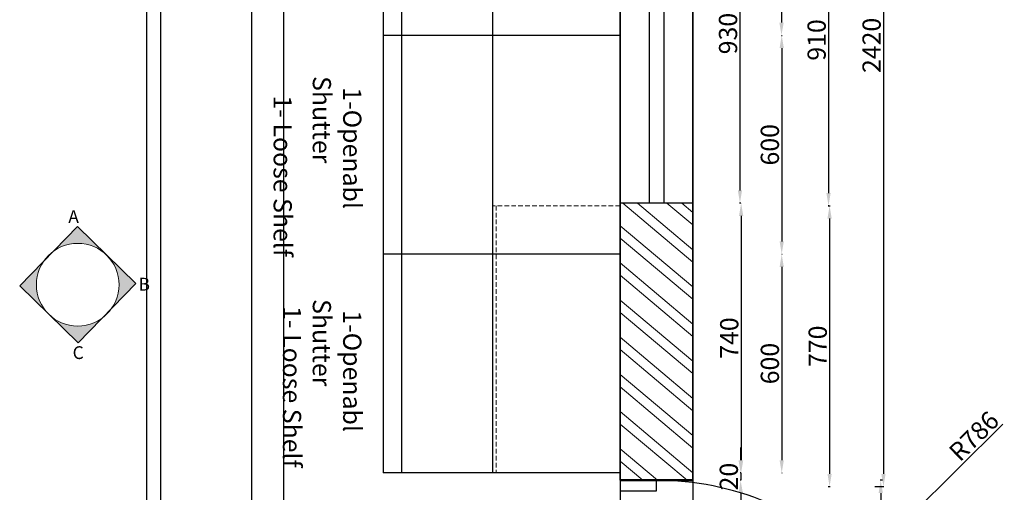
# Model space of a CAD drawing. Units: millimetres. Extents: x 407065 to 421840, y 1168257 to 1177792.
# Tile 8 of 17: x 409176 to 411879, y 1174685 to 1175981. Entities that reach past the tile are written whole.
import ezdxf

# ---------------------------------------------------------------- set-up
doc = ezdxf.new("R2010")
doc.units = ezdxf.units.MM
doc.linetypes.add('DASHED', pattern=[19.05, 12.7, -6.35])
for name, color, linetype, lineweight in [('A-ANNO-DIMS', 6, 'Continuous', 18), ('A-ANNO-SYMB', 6, 'Continuous', 18), ('A-ANNO-TEXT', 30, 'Continuous', 18), ('A-DOOR', 4, 'Continuous', 25), ('A-FURN', 3, 'Continuous', 25), ('A-FURN-HIDN', 7, 'DASHED', 18), ('A-WALL', 7, 'Continuous', 50), ('A-WALL-PATT', 8, 'Continuous', 13)]:
    doc.layers.add(name, color=color, linetype=linetype, lineweight=lineweight)
doc.styles.get("Standard").update_dxf_attribs({"font": 'arial.ttf'})
doc.dimstyles.new('ISO-25', dxfattribs={"dimtxt": 50, "dimasz": 35, "dimexe": 1.25, "dimexo": 0.625, "dimtad": 1, "dimdec": 1, "dimtxsty": 'Standard', "dimcen": 35, "dimadec": 0, "dimazin": 0, "dimtfac": 1, "dimtdec": 1, "dimtmove": 0, "dimatfit": 3, "dimfxl": 1, "dimarcsym": 0})

# ---------------------------------------------------------------- blocks, each defined once
blk = doc.blocks.new('*D21')
at = {"layer": 'A-ANNO-DIMS', "color": 0, "lineweight": -2, "transparency": 16777216}
for p, q in [((411156.1, 1176407.8), (411152.2, 1176407.8)), ((411153.4, 1176372.8), (411153.4, 1175512.8)), ((411156.1, 1175477.8), (411152.2, 1175477.8))]:
    blk.add_line(p, q, dxfattribs=at)
at = {"layer": 'A-ANNO-DIMS', "color": 0, "transparency": 16777216}
for points in [[(411147.6, 1176372.8), (411159.2, 1176372.8), (411153.4, 1176407.8)], [(411147.6, 1175512.8), (411159.2, 1175512.8), (411153.4, 1175477.8)]]:
    blk.add_solid(points, dxfattribs=at)
at = {"layer": 'Defpoints', "color": 0, "transparency": 16777216}
for p in [(411156.7, 1176407.8), (411153.4, 1175477.8), (411156.7, 1175477.8)]:
    blk.add_point(p, dxfattribs=at)
at = {"layer": 'A-ANNO-DIMS', "color": 0, "transparency": 16777216, "insert": (411127.2, 1175942.8), "char_height": 50, "attachment_point": 5, "rotation": 90}
blk.add_mtext('930', dxfattribs=at)
blk = doc.blocks.new('*D22')
at = {"layer": 'A-ANNO-DIMS', "color": 0, "lineweight": -2, "transparency": 16777216}
for p, q in [((411157.3, 1175477.8), (411157.9, 1175477.8)), ((411156.7, 1175442.8), (411156.7, 1174772.8)), ((411157.3, 1174737.8), (411157.9, 1174737.8))]:
    blk.add_line(p, q, dxfattribs=at)
at = {"layer": 'A-ANNO-DIMS', "color": 0, "transparency": 16777216}
for points in [[(411150.8, 1175442.8), (411162.5, 1175442.8), (411156.7, 1175477.8)], [(411150.8, 1174772.8), (411162.5, 1174772.8), (411156.7, 1174737.8)]]:
    blk.add_solid(points, dxfattribs=at)
at = {"layer": 'Defpoints', "color": 0, "transparency": 16777216}
for p in [(411156.7, 1175477.8), (411156.7, 1174737.8), (411156.7, 1174737.8)]:
    blk.add_point(p, dxfattribs=at)
at = {"layer": 'A-ANNO-DIMS', "color": 0, "transparency": 16777216, "insert": (411130.5, 1175107.8), "char_height": 50, "attachment_point": 5, "rotation": 90}
blk.add_mtext('740', dxfattribs=at)
blk = doc.blocks.new('*D23')
at = {"layer": 'A-ANNO-DIMS', "color": 0, "lineweight": -2, "transparency": 16777216}
for p, q in [((411155.4, 1174772.8), (411155.4, 1174807.8)), ((411156.1, 1174737.8), (411154.2, 1174737.8)), ((411155.4, 1174737.8), (411155.4, 1174717.8)), ((411156.1, 1174717.8), (411154.2, 1174717.8)), ((411155.4, 1174682.8), (411155.4, 1174647.8))]:
    blk.add_line(p, q, dxfattribs=at)
at = {"layer": 'A-ANNO-DIMS', "color": 0, "transparency": 16777216}
for points in [[(411149.6, 1174772.8), (411161.3, 1174772.8), (411155.4, 1174737.8)], [(411149.6, 1174682.8), (411161.3, 1174682.8), (411155.4, 1174717.8)]]:
    blk.add_solid(points, dxfattribs=at)
at = {"layer": 'Defpoints', "color": 0, "transparency": 16777216}
for p in [(411156.7, 1174737.8), (411155.4, 1174717.8), (411156.7, 1174717.8)]:
    blk.add_point(p, dxfattribs=at)
at = {"layer": 'A-ANNO-DIMS', "color": 0, "transparency": 16777216, "insert": (411129.3, 1174727.8), "char_height": 50, "attachment_point": 5, "rotation": 90}
blk.add_mtext('20', dxfattribs=at)
blk = doc.blocks.new('*D24')
at = {"layer": 'A-ANNO-DIMS', "color": 0, "lineweight": -2, "transparency": 16777216}
for p, q in [((411545.1, 1174717.8), (411538.7, 1174717.8)), ((411539.9, 1174682.8), (411539.9, 1173927.8)), ((411545.1, 1173892.8), (411538.7, 1173892.8))]:
    blk.add_line(p, q, dxfattribs=at)
at = {"layer": 'A-ANNO-DIMS', "color": 0, "transparency": 16777216}
for points in [[(411534.1, 1174682.8), (411545.8, 1174682.8), (411539.9, 1174717.8)], [(411534.1, 1173927.8), (411545.8, 1173927.8), (411539.9, 1173892.8)]]:
    blk.add_solid(points, dxfattribs=at)
at = {"layer": 'Defpoints', "color": 0, "transparency": 16777216}
for p in [(411545.8, 1174717.8), (411539.9, 1173892.8), (411545.8, 1173892.8)]:
    blk.add_point(p, dxfattribs=at)
at = {"layer": 'A-ANNO-DIMS', "color": 0, "transparency": 16777216, "insert": (411513.8, 1174305.3), "char_height": 50, "attachment_point": 5, "rotation": 90}
blk.add_mtext('825', dxfattribs=at)
blk = doc.blocks.new('*D28')
at = {"layer": 'A-ANNO-DIMS', "color": 0, "lineweight": -2, "transparency": 16777216}
for p, q in [((411267.4, 1176487.8), (411268.8, 1176487.8)), ((411267.5, 1176452.8), (411267.5, 1175972.8)), ((411267.4, 1175937.8), (411268.8, 1175937.8))]:
    blk.add_line(p, q, dxfattribs=at)
at = {"layer": 'A-ANNO-DIMS', "color": 0, "transparency": 16777216}
for points in [[(411261.7, 1176452.8), (411273.4, 1176452.8), (411267.5, 1176487.8)], [(411261.7, 1175972.8), (411273.4, 1175972.8), (411267.5, 1175937.8)]]:
    blk.add_solid(points, dxfattribs=at)
at = {"layer": 'Defpoints', "color": 0, "transparency": 16777216}
for p in [(411266.8, 1176487.8), (411266.8, 1175937.8), (411267.5, 1175937.8)]:
    blk.add_point(p, dxfattribs=at)
at = {"layer": 'A-ANNO-DIMS', "color": 0, "transparency": 16777216, "insert": (411241.4, 1176212.8), "char_height": 50, "attachment_point": 5, "rotation": 90}
blk.add_mtext('550', dxfattribs=at)
blk = doc.blocks.new('*D29')
at = {"layer": 'A-ANNO-DIMS', "color": 0, "lineweight": -2, "transparency": 16777216}
for p, q in [((411268.7, 1175937.8), (411269.4, 1175937.8)), ((411268.1, 1175902.8), (411268.1, 1175372.8)), ((411268.7, 1175337.8), (411269.4, 1175337.8))]:
    blk.add_line(p, q, dxfattribs=at)
at = {"layer": 'A-ANNO-DIMS', "color": 0, "transparency": 16777216}
for points in [[(411262.3, 1175902.8), (411273.9, 1175902.8), (411268.1, 1175937.8)], [(411262.3, 1175372.8), (411273.9, 1175372.8), (411268.1, 1175337.8)]]:
    blk.add_solid(points, dxfattribs=at)
at = {"layer": 'Defpoints', "color": 0, "transparency": 16777216}
for p in [(411268.1, 1175937.8), (411268.1, 1175337.8), (411268.1, 1175337.8)]:
    blk.add_point(p, dxfattribs=at)
at = {"layer": 'A-ANNO-DIMS', "color": 0, "transparency": 16777216, "insert": (411242, 1175637.8), "char_height": 50, "attachment_point": 5, "rotation": 90}
blk.add_mtext('600', dxfattribs=at)
blk = doc.blocks.new('*D30')
at = {"layer": 'A-ANNO-DIMS', "color": 0, "lineweight": -2, "transparency": 16777216}
for p, q in [((411268.7, 1175337.8), (411269.4, 1175337.8)), ((411268.1, 1175302.8), (411268.1, 1174772.8)), ((411268.7, 1174737.8), (411269.4, 1174737.8))]:
    blk.add_line(p, q, dxfattribs=at)
at = {"layer": 'A-ANNO-DIMS', "color": 0, "transparency": 16777216}
for points in [[(411262.3, 1175302.8), (411273.9, 1175302.8), (411268.1, 1175337.8)], [(411262.3, 1174772.8), (411273.9, 1174772.8), (411268.1, 1174737.8)]]:
    blk.add_solid(points, dxfattribs=at)
at = {"layer": 'Defpoints', "color": 0, "transparency": 16777216}
for p in [(411268.1, 1175337.8), (411268.1, 1174737.8), (411268.1, 1174737.8)]:
    blk.add_point(p, dxfattribs=at)
at = {"layer": 'A-ANNO-DIMS', "color": 0, "transparency": 16777216, "insert": (411242, 1175037.8), "char_height": 50, "attachment_point": 5, "rotation": 90}
blk.add_mtext('600', dxfattribs=at)
blk = doc.blocks.new('*D32')
at = {"layer": 'A-ANNO-DIMS', "color": 0, "lineweight": -2, "transparency": 16777216}
for p, q in [((411397.2, 1176380.3), (411395.3, 1176380.3)), ((411396.6, 1176345.3), (411396.6, 1175505.3)), ((411397.2, 1175470.3), (411395.3, 1175470.3))]:
    blk.add_line(p, q, dxfattribs=at)
at = {"layer": 'A-ANNO-DIMS', "color": 0, "transparency": 16777216}
for points in [[(411390.8, 1176345.3), (411402.4, 1176345.3), (411396.6, 1176380.3)], [(411390.8, 1175505.3), (411402.4, 1175505.3), (411396.6, 1175470.3)]]:
    blk.add_solid(points, dxfattribs=at)
at = {"layer": 'Defpoints', "color": 0, "transparency": 16777216}
for p in [(411397.8, 1176380.3), (411396.6, 1175470.3), (411397.8, 1175470.3)]:
    blk.add_point(p, dxfattribs=at)
at = {"layer": 'A-ANNO-DIMS', "color": 0, "transparency": 16777216, "insert": (411370.4, 1175925.3), "char_height": 50, "attachment_point": 5, "rotation": 90}
blk.add_mtext('910', dxfattribs=at)
blk = doc.blocks.new('*D33')
at = {"layer": 'A-ANNO-DIMS', "color": 0, "lineweight": -2, "transparency": 16777216}
for p, q in [((411396, 1175470.3), (411400.8, 1175470.3)), ((411399.5, 1175435.3), (411399.5, 1174735.3)), ((411396, 1174700.3), (411400.8, 1174700.3))]:
    blk.add_line(p, q, dxfattribs=at)
at = {"layer": 'A-ANNO-DIMS', "color": 0, "transparency": 16777216}
for points in [[(411393.7, 1175435.3), (411405.3, 1175435.3), (411399.5, 1175470.3)], [(411393.7, 1174735.3), (411405.3, 1174735.3), (411399.5, 1174700.3)]]:
    blk.add_solid(points, dxfattribs=at)
at = {"layer": 'Defpoints', "color": 0, "transparency": 16777216}
for p in [(411395.3, 1175470.3), (411395.3, 1174700.3), (411399.5, 1174700.3)]:
    blk.add_point(p, dxfattribs=at)
at = {"layer": 'A-ANNO-DIMS', "color": 0, "transparency": 16777216, "insert": (411373.4, 1175085.3), "char_height": 50, "attachment_point": 5, "rotation": 90}
blk.add_mtext('770', dxfattribs=at)
blk = doc.blocks.new('*D34')
at = {"layer": 'A-ANNO-DIMS', "color": 0, "lineweight": -2, "transparency": 16777216}
for p, q in [((411523.7, 1177120.3), (411548.7, 1177120.3)), ((411547.4, 1177085.3), (411547.4, 1174735.3)), ((411523.7, 1174700.3), (411548.7, 1174700.3))]:
    blk.add_line(p, q, dxfattribs=at)
at = {"layer": 'A-ANNO-DIMS', "color": 0, "transparency": 16777216}
for points in [[(411541.6, 1177085.3), (411553.3, 1177085.3), (411547.4, 1177120.3)], [(411541.6, 1174735.3), (411553.3, 1174735.3), (411547.4, 1174700.3)]]:
    blk.add_solid(points, dxfattribs=at)
at = {"layer": 'Defpoints', "color": 0, "transparency": 16777216}
for p in [(411523.1, 1177120.3), (411523.1, 1174700.3), (411547.4, 1174700.3)]:
    blk.add_point(p, dxfattribs=at)
at = {"layer": 'A-ANNO-DIMS', "color": 0, "transparency": 16777216, "insert": (411521.3, 1175910.3), "char_height": 50, "attachment_point": 5, "rotation": 90}
blk.add_mtext('2420', dxfattribs=at)
blk = doc.blocks.new('*D169')
at = {"layer": 'A-ANNO-DIMS', "color": 0, "lineweight": -2, "transparency": 16777216}
for p, q in [((410824.3, 1174717.2), (410824.3, 1172896.5)), ((411024.3, 1174717.2), (411024.3, 1172896.5)), ((410859.3, 1172897.8), (410989.3, 1172897.8))]:
    blk.add_line(p, q, dxfattribs=at)
at = {"layer": 'A-ANNO-DIMS', "color": 0, "transparency": 16777216}
for points in [[(410859.3, 1172903.6), (410859.3, 1172892), (410824.3, 1172897.8)], [(410989.3, 1172903.6), (410989.3, 1172892), (411024.3, 1172897.8)]]:
    blk.add_solid(points, dxfattribs=at)
at = {"layer": 'Defpoints', "color": 0, "transparency": 16777216}
for p in [(410824.3, 1174717.8), (411024.3, 1174717.8), (411024.3, 1172897.8)]:
    blk.add_point(p, dxfattribs=at)
at = {"layer": 'A-ANNO-DIMS', "color": 0, "transparency": 16777216, "insert": (410924.3, 1172923.9), "char_height": 50, "attachment_point": 5}
blk.add_mtext('200', dxfattribs=at)
blk = doc.blocks.new('*D184')
at = {"layer": 'A-ANNO-DIMS', "color": 0, "lineweight": -2, "transparency": 16777216}
for p, q in [((409524, 1176776.8), (409524, 1172896.5)), ((409900.3, 1176764.7), (409900.3, 1172896.5)), ((409559, 1172897.8), (409865.3, 1172897.8))]:
    blk.add_line(p, q, dxfattribs=at)
at = {"layer": 'A-ANNO-DIMS', "color": 0, "transparency": 16777216}
for points in [[(409559, 1172903.6), (409559, 1172892), (409524, 1172897.8)], [(409865.3, 1172903.6), (409865.3, 1172892), (409900.3, 1172897.8)]]:
    blk.add_solid(points, dxfattribs=at)
at = {"layer": 'Defpoints', "color": 0, "transparency": 16777216}
for p in [(409524, 1176777.5), (409900.3, 1176765.3), (409900.3, 1172897.8)]:
    blk.add_point(p, dxfattribs=at)
at = {"layer": 'A-ANNO-DIMS', "color": 0, "transparency": 16777216, "insert": (409712.1, 1172924), "char_height": 50, "attachment_point": 5}
blk.add_mtext('376.24', dxfattribs=at)
blk = doc.blocks.new('*D185')
at = {"layer": 'A-ANNO-DIMS', "color": 0, "lineweight": -2, "transparency": 16777216}
for p, q in [((409562.3, 1176698.3), (409562.3, 1172896.5)), ((409812.5, 1176698.3), (409812.5, 1172896.5)), ((409597.3, 1172897.8), (409777.5, 1172897.8))]:
    blk.add_line(p, q, dxfattribs=at)
at = {"layer": 'A-ANNO-DIMS', "color": 0, "transparency": 16777216}
for points in [[(409597.3, 1172903.6), (409597.3, 1172892), (409562.3, 1172897.8)], [(409777.5, 1172903.6), (409777.5, 1172892), (409812.5, 1172897.8)]]:
    blk.add_solid(points, dxfattribs=at)
at = {"layer": 'Defpoints', "color": 0, "transparency": 16777216}
for p in [(409562.3, 1176698.9), (409812.5, 1176698.9), (409812.5, 1172897.8)]:
    blk.add_point(p, dxfattribs=at)
at = {"layer": 'A-ANNO-DIMS', "color": 0, "transparency": 16777216, "insert": (409687.4, 1172923.9), "char_height": 50, "attachment_point": 5}
blk.add_mtext('250.25', dxfattribs=at)
blk = doc.blocks.new('*D233')
at = {"layer": 'A-ANNO-DIMS', "color": 0, "lineweight": -2, "transparency": 16777216}
for p, q in [((411875.5, 1174871.8), (411508.2, 1174508.9)), ((410924.3, 1173931.9), (411483.3, 1174484.3))]:
    blk.add_line(p, q, dxfattribs=at)
at = {"layer": 'A-ANNO-DIMS', "color": 0, "transparency": 16777216}
blk.add_solid([(411504.1, 1174513.1), (411512.3, 1174504.8), (411483.3, 1174484.3)], dxfattribs=at)
at = {"layer": 'Defpoints', "color": 0, "transparency": 16777216}
for p in [(411483.3, 1174484.3), (410924.3, 1173931.9)]:
    blk.add_point(p, dxfattribs=at)
at = {"layer": 'A-ANNO-DIMS', "color": 0, "transparency": 16777216, "insert": (411800.3, 1174834.4), "char_height": 50, "attachment_point": 5, "rotation": 44.6617}
blk.add_mtext('R786', dxfattribs=at)

msp = doc.modelspace()

# ---------------------------------------------------------------- hatches: boundary and pattern name
at = {"layer": 'A-ANNO-SYMB'}
h = msp.add_hatch(color=256, dxfattribs=at)
h.dxf.hatch_style = 1
h.paths.add_polyline_path([(409334.3181, 1175413.4673), (409267.9619, 1175345.3591, -0.367382348), (409414.5012, 1175335.3468)])
h = msp.add_hatch(color=256, dxfattribs=at)
h.dxf.hatch_style = 1
h.paths.add_polyline_path([(409494.6843, 1175257.2263), (409414.5012, 1175335.3468, -0.202300593), (409448.7793, 1175254.0934, -0.153661385), (409428.328, 1175189.1181)])
h = msp.add_hatch(color=256, dxfattribs=at)
h.dxf.hatch_style = 1
h.paths.add_polyline_path([(409242.3477, 1175319.0687), (409175.9915, 1175250.9604), (409256.1746, 1175172.8399, -0.202300593), (409221.8965, 1175254.0934, -0.153661385)])
h = msp.add_hatch(color=256, dxfattribs=at)
h.dxf.hatch_style = 1
h.paths.add_polyline_path([(409402.7139, 1175162.8277, -0.367382348), (409256.1746, 1175172.8399), (409336.3576, 1175094.7194)])
at = {"layer": 'A-WALL-PATT'}
h = msp.add_hatch(dxfattribs=at)
h.set_pattern_fill('ANSI32', color=256, scale=8.2, angle=95)
h.paths.add_polyline_path([(411024.3133, 1175477.7952), (410824.3133, 1175477.7952), (410824.3133, 1174717.7952), (410924.3133, 1174717.7952), (411024.3133, 1174717.7952)])

# ---------------------------------------------------------------- linework, layer by layer
at = {"layer": 'A-ANNO-SYMB'}
msp.add_lwpolyline([(409334.3181, 1175413.4673), (409494.6843, 1175257.2263), (409336.3576, 1175094.7194), (409175.9915, 1175250.9604)], close=True, dxfattribs=at)
msp.add_circle((409335.3379, 1175254.0934), 113.4414, dxfattribs=at)
at = {"layer": 'A-DOOR'}
msp.add_arc((410924.3133, 1173931.8713), 785.9239, 359.2709558, 90, dxfattribs=at)
at = {"layer": 'A-FURN'}
for p, q in [((411024.3133, 1174717.7952), (411024.3133, 1177437.7952)), ((410174.3133, 1177137.7952), (410174.3133, 1174737.7952)), ((410224.3133, 1177137.7952), (410224.3133, 1174737.7952)), ((410474.3133, 1177137.7952), (410474.3133, 1174737.7952)), ((410824.3133, 1177137.7952), (410824.3133, 1174717.7952)), ((410824.3133, 1174717.7952), (410824.3133, 1177137.7952)), ((411024.3133, 1177137.7952), (411024.3133, 1174717.7952)), ((410904.3133, 1176407.7952), (410904.3133, 1175477.7952)), ((410944.3133, 1176407.7952), (410944.3133, 1175477.7952)), ((410824.3133, 1175937.7952), (410174.3133, 1175937.7952)), ((410824.3133, 1175337.7952), (410174.3133, 1175337.7952)), ((410824.3133, 1174737.7952), (410174.3133, 1174737.7952))]:
    msp.add_line(p, q, dxfattribs=at)
for points in [[(410824.3133, 1176407.7952), (411024.3133, 1176407.7952), (411024.3133, 1175477.7952), (410824.3133, 1175477.7952)], [(410924.3133, 1174717.7952), (410824.3133, 1174717.7952), (410824.3133, 1174688.7192), (410924.3133, 1174688.7192)]]:
    msp.add_lwpolyline(points, close=True, dxfattribs=at)
at = {"layer": 'A-FURN-HIDN'}
for p, q in [((410824.3133, 1175470.5608), (410474.3133, 1175470.5608)), ((410484.3133, 1175470.5608), (410484.3133, 1174737.7952))]:
    msp.add_line(p, q, dxfattribs=at)
at = {"layer": 'A-WALL'}
msp.add_line((411024.3133, 1174717.7952), (410824.3133, 1174717.7952), dxfattribs=at)

# ---------------------------------------------------------------- texts
at = {"layer": 'A-ANNO-TEXT', "char_height": 50, "attachment_point": 1, "rotation": 270}
for s, width, insert in [('  1-Openabl Shutter', 520.083559, (410113.9732, 1175826.174)), ('1- Loose Shelf', 482.488338, (409923.0821, 1175773.0385)), ('  1-Openabl Shutter', 513.083996, (410113.9732, 1175214.5945)), ('1- Loose Shelf', 485.449025, (409948.7606, 1175195.2742))]:
    msp.add_mtext_dynamic_manual_height_columns(s, width=width, gutter_width=12.5, heights=[0], dxfattribs=dict(at, insert=insert))
at = {"layer": 'A-ANNO-TEXT', "char_height": 35, "attachment_point": 1}
for s, insert in [('A', (409309.404, 1175458.3772)), ('B', (409502.3558, 1175272.9916)), ('C', (409321.3305, 1175085.2406))]:
    msp.add_mtext_dynamic_manual_height_columns(s, width=382.409863, gutter_width=12.5, heights=[0], dxfattribs=dict(at, insert=insert))

# ---------------------------------------------------------------- dimensions: what is measured, and where the dimension line sits
at = {"layer": 'A-ANNO-DIMS'}
for base, p1, p2, picture, middle in [((411547.4266, 1174700.2952), (411523.1043, 1177120.2952), (411523.1043, 1174700.2952), '*D34', (411521.2729, 1175910.2952)), ((411267.522, 1175937.7952), (411266.8192, 1176487.7952), (411266.8192, 1175937.7952), '*D28', (411241.3684, 1176212.7952)), ((411153.4065, 1175477.7952), (411156.6757, 1176407.7952), (411156.6757, 1175477.7952), '*D21', (411127.2358, 1175942.7952)), ((411396.5925, 1175470.2952), (411397.8425, 1176380.2952), (411397.8425, 1175470.2952), '*D32', (411370.4388, 1175925.2952)), ((411268.1081, 1175337.7952), (411268.1081, 1175937.7952), (411268.1081, 1175337.7952), '*D29', (411241.9544, 1175637.7952)), ((411156.6757, 1174737.7952), (411156.6757, 1175477.7952), (411156.6757, 1174737.7952), '*D22', (411130.522, 1175107.7952)), ((411399.5092, 1174700.2952), (411395.3425, 1175470.2952), (411395.3425, 1174700.2952), '*D33', (411373.3555, 1175085.2952)), ((411268.1081, 1174737.7952), (411268.1081, 1175337.7952), (411268.1081, 1174737.7952), '*D30', (411241.9544, 1175037.7952)), ((411539.9266, 1173892.7952), (411545.7599, 1174717.7952), (411545.7599, 1173892.7952), '*D24', (411513.7729, 1174305.2952))]:
    dim = msp.add_linear_dim(base=base, p1=p1, p2=p2, angle=90, dimstyle='ISO-25', override={"dimclrd": 0, "dimclre": 0, "dimclrt": 0}, dxfattribs=at)
    dim.commit()
    dim.dimension.update_dxf_attribs({"geometry": picture, "text_midpoint": middle})
for base, p1, p2, override, picture, middle in [((409900.2591, 1172897.7952), (409524.0157, 1176777.4536), (409900.2591, 1176765.2756), {"dimdec": 2, "dimlfac": 1, "dimrnd": 0, "dimzin": 0, "dimdsep": 46, "dimlunit": 2}, '*D184', (409712.1374, 1172923.9659)), ((409812.5157, 1172897.7952), (409562.2649, 1176698.8834), (409812.5157, 1176698.8834), {"dimdec": 2, "dimlfac": 1, "dimrnd": 0, "dimzin": 0, "dimdsep": 46, "dimlunit": 2}, '*D185', (409687.3903, 1172923.9489)), ((411024.3133, 1172897.7952), (410824.3133, 1174717.7952), (411024.3133, 1174717.7952), {"dimdec": 0, "dimlfac": 1, "dimrnd": 0, "dimzin": 0, "dimdsep": 46, "dimlunit": 2}, '*D169', (410924.3133, 1172923.9489))]:
    dim = msp.add_linear_dim(base=base, p1=p1, p2=p2, dimstyle='ISO-25', override=override, dxfattribs=at)
    dim.commit()
    dim.dimension.update_dxf_attribs({"geometry": picture, "text_midpoint": middle})
dim = msp.add_radius_dim(center=(410924.3133, 1173931.8713), mpoint=(411483.3166, 1174484.3129), dimstyle='ISO-25', override={"dimdec": 0, "dimlfac": 1, "dimrnd": 0, "dimzin": 0, "dimdsep": 46, "dimlunit": 2}, dxfattribs=at)
dim.commit()
dim.dimension.update_dxf_attribs({"geometry": '*D233', "text_midpoint": (411818.7186, 1174815.7779), "dimtype": 164})
dim = msp.add_linear_dim(base=(411155.4257, 1174717.7952), p1=(411156.6757, 1174737.7952), p2=(411156.6757, 1174717.7952), angle=90, dimstyle='ISO-25', override={"dimclrd": 0, "dimclre": 0, "dimclrt": 0}, dxfattribs=at)
dim.commit()
dim.dimension.update_dxf_attribs({"geometry": '*D23', "text_midpoint": (411155.4257, 1174727.7952), "dimtype": 160})

doc.saveas('drawing.dxf')
